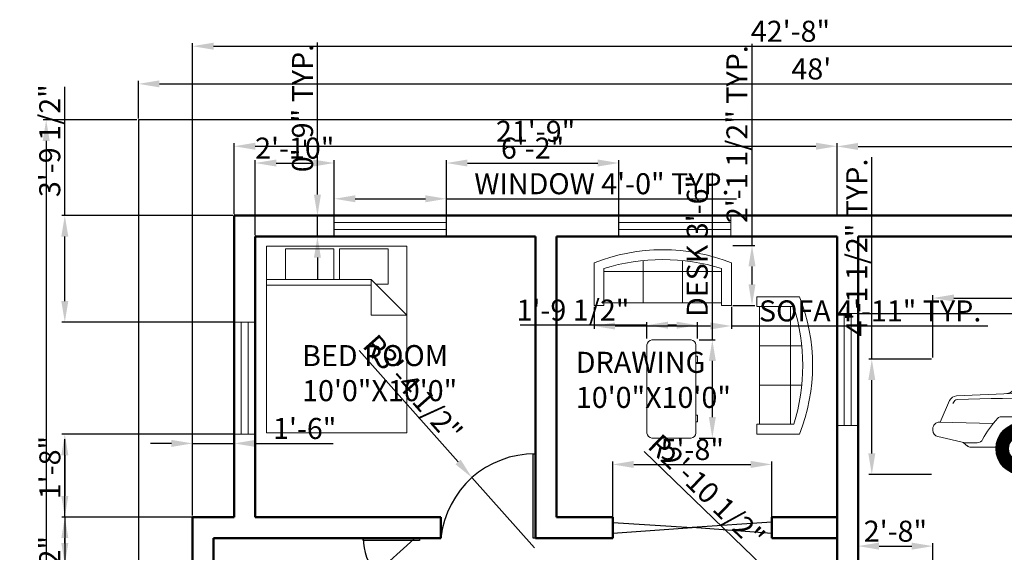
# Model space of a CAD drawing. Units: inches. Extents: x 2059616 to 2060276, y 889994 to 890582.
# Tile 3 of 4: x 2059616 to 2060037, y 890354 to 890582. Entities that reach past the tile are written whole.
import ezdxf

# ---------------------------------------------------------------- set-up
doc = ezdxf.new("R2010")
doc.units = ezdxf.units.IN
for name, color, linetype, lineweight in [('A-ANNO-DIMS', 2, 'Continuous', 18), ('A-AREA-IDEN', 7, 'Continuous', 25), ('A-DOOR', 3, 'Continuous', 25), ('A-FURN', 8, 'Continuous', 18), ('A-GLAZ', 4, 'Continuous', 18), ('A-SITE-VEHC', 8, 'Continuous', 18), ('A-WALL', 7, 'Continuous', 50), ('C-PROP', 7, 'Continuous', 25)]:
    doc.layers.add(name, color=color, linetype=linetype, lineweight=lineweight)
doc.styles.get("Standard").update_dxf_attribs({"font": 'arial.ttf'})
doc.dimstyles.new('ISO-25', dxfattribs={"dimtxt": 9, "dimasz": 9, "dimexe": 1.25, "dimexo": 0.625, "dimtad": 1, "dimdec": 1, "dimrnd": 9, "dimlunit": 3, "dimtxsty": 'Standard', "dimcen": 2.5, "dimadec": 0, "dimazin": 0, "dimtfac": 1, "dimtdec": 1, "dimtmove": 0, "dimatfit": 3, "dimfxl": 1, "dimarcsym": 0})

# ---------------------------------------------------------------- blocks, each defined once
blk = doc.blocks.new('*D1')
at = {"layer": 'A-ANNO-DIMS', "color": 0, "lineweight": -2, "transparency": 16777216}
for p, q in [((2059666.76, 890539.47), (2059666.76, 890555.48)), ((2059675.76, 890554.23), (2060233.76, 890554.23)), ((2060242.76, 890539.47), (2060242.76, 890555.48))]:
    blk.add_line(p, q, dxfattribs=at)
at = {"layer": 'A-ANNO-DIMS', "color": 0, "transparency": 16777216}
for points in [[(2059675.76, 890555.73), (2059675.76, 890552.73), (2059666.76, 890554.23)], [(2060233.76, 890555.73), (2060233.76, 890552.73), (2060242.76, 890554.23)]]:
    blk.add_solid(points, dxfattribs=at)
at = {"layer": 'Defpoints', "color": 0, "transparency": 16777216}
for p in [(2060242.76, 890554.23), (2059666.76, 890538.85), (2060242.76, 890538.85)]:
    blk.add_point(p, dxfattribs=at)
at = {"layer": 'A-ANNO-DIMS', "color": 0, "transparency": 16777216, "insert": (2059954.76, 890559.45), "char_height": 9, "attachment_point": 5}
blk.add_mtext("48'", dxfattribs=at)
blk = doc.blocks.new('*D2')
at = {"layer": 'A-ANNO-DIMS', "color": 0, "lineweight": -2, "transparency": 16777216}
for p, q in [((2059666.14, 890538.85), (2059626.05, 890538.85)), ((2059627.3, 890529.85), (2059627.3, 890091.85)), ((2059666.14, 890082.85), (2059626.05, 890082.85))]:
    blk.add_line(p, q, dxfattribs=at)
at = {"layer": 'A-ANNO-DIMS', "color": 0, "transparency": 16777216}
for points in [[(2059625.8, 890529.85), (2059628.8, 890529.85), (2059627.3, 890538.85)], [(2059625.8, 890091.85), (2059628.8, 890091.85), (2059627.3, 890082.85)]]:
    blk.add_solid(points, dxfattribs=at)
at = {"layer": 'Defpoints', "color": 0, "transparency": 16777216}
for p in [(2059666.76, 890538.85), (2059627.3, 890082.85), (2059666.76, 890082.85)]:
    blk.add_point(p, dxfattribs=at)
at = {"layer": 'A-ANNO-DIMS', "color": 0, "transparency": 16777216, "insert": (2059622.08, 890310.85), "char_height": 9, "attachment_point": 5, "rotation": 90}
blk.add_mtext('38\'-3"', dxfattribs=at)
blk = doc.blocks.new('Car - sedan  side')
for p, q in [((-139.53, 35.99), (-129.64, 47.91)), ((-128.57, 32.64), (-121.22, 48.02)), ((-77.81, 49.34), (-126.58, 49.34)), ((-74.7, 48.02), (-121.22, 48.02)), ((-120.32, 34.67), (-115.67, 48.02)), ((-115.4, 34.67), (-111.74, 48.02)), ((-97.55, 47.3), (-111.94, 47.3)), ((-94.41, 34.67), (-97.73, 48.02)), ((-93.72, 34.67), (-97.04, 48.02)), ((-93.03, 34.67), (-96.34, 48.02)), ((-76.26, 47.3), (-96.16, 47.3)), ((-61.08, 34.66), (-76.26, 47.3)), ((-60.02, 34.65), (-76.07, 48.02)), ((-56.87, 35.13), (-75.48, 48.59)), ((-58.54, 34.93), (-74.99, 48.02)), ((-140.23, 34.67), (-163.88, 33.56)), ((-62.28, 34.67), (-140.23, 34.67)), ((-93.72, 19.62), (-93.72, 34.67)), ((-62.28, 34.67), (-60.02, 34.65)), ((-60.02, 34.65), (-58.54, 34.93)), ((-57.97, 31.61), (-60.02, 34.65)), ((-57.21, 35.38), (-58.54, 34.93)), ((-54.93, 34.4), (-8.75, 29.8)), ((-170.93, 22.32), (-166.81, 31.56)), ((-164.57, 31.6), (-165.48, 30.35)), ((-130.39, 24.63), (-128.57, 32.64)), ((-57.97, 19.62), (-57.97, 31.61)), ((-4.21, 24.18), (-5.42, 27.27)), ((-148.26, 21.7), (-171.11, 22.33)), ((-128.78, 24.63), (-144.79, 24.63)), ((-36.97, 24.38), (-34.94, 24.38)), ((-174, 19.51), (-174, 18.91)), ((-47.2, 19.62), (-125.23, 19.62)), ((-93.72, 12.14), (-93.72, 19.62)), ((-57.97, 12.14), (-57.97, 19.62)), ((0, 19.62), (-24.7, 19.62)), ((-160.12, 13.48), (-171.81, 16.16)), ((-159.22, 12.14), (-161.08, 13.7)), ((-155.01, 13.48), (-160.12, 13.48)), ((-51.4, 9.89), (-49.69, 15.14)), ((-4.23, 13.19), (-20.72, 13.19)), ((-9.5, 13.19), (-14.1, 10.2)), ((-3.22, 13.59), (-1.77, 14.97)), ((-147.03, 11.6), (-157.73, 11.6)), ((-120.62, 9.03), (-125.23, 9.03)), ((-50.67, 12.14), (-123.32, 12.14)), ((-45.76, 9.03), (-120.62, 9.03)), ((-94.21, 9.03), (-94.21, 12.14)), ((-58.39, 9.03), (-58.39, 12.14)), ((-20.36, 11.06), (-24.06, 9.44)), ((-18.83, 10.42), (-19.11, 10.76)), ((-14.68, 10.03), (-18.01, 10.03))]:
    blk.add_line(p, q)
at = {"const_width": 5.49}
for points in [[(-127.8, 11, -1), (-144.3, 11, -1)], [(-26.69, 11, -1), (-43.19, 11, -1)]]:
    blk.add_lwpolyline(points, format="xyb", close=True, dxfattribs=at)
for centre, radius in [((-136.05, 11), 11), ((-34.94, 11), 11), ((-136.05, 11), 5.51), ((-34.94, 11), 5.51)]:
    blk.add_circle(centre, radius)
for centre, radius, start, end in [((-126.58, 45.38), 3.97, 90, 140.3029), ((-77.81, 45.38), 3.97, 54.135, 90), ((-142.58, 38.53), 3.97, 272.6827, 320.3029), ((-54.54, 38.35), 3.97, 234.135, 264.3123), ((-163.72, 30.18), 3.38, 92.6827, 155.9736), ((-163.62, 30.91), 1.17, 91.491, 143.9553), ((-118.51, -1702.12), 1734.79, 86.34698, 91.49105), ((-9.15, 25.82), 4, 21.3107, 84.3123), ((-171.18, 19.51), 2.82, 88.4193, 180), ((-118.09, -2.78), 38.85, 136.3964, 152.9097), ((-144.79, 22.64), 1.98, 90, 136.3964), ((-128.78, 22.64), 1.98, 28.1371, 90), ((-157.14, 7.48), 34.14, 6.5135, 28.1371), ((-36.97, 11), 13.38, 90, 161.9732), ((-34.94, 11), 13.38, 13.5864, 90), ((0.9, 26.18), 5.49, 201.3107, 247.7048), ((-1.92, 19.3), 1.94, 325.3744, 67.7048), ((-171.18, 18.91), 2.82, 180, 257.0905), ((2.46, 16.28), 3.37, 145.3744, 172.3839), ((-155.01, 16.1), 2.62, 270, 332.9097), ((-20.72, 14.43), 1.24, 193.5864, 270), ((-4.23, 14.65), 1.46, 270, 313.7173), ((-3.82, 17.12), 2.96, 313.7173, 352.3839), ((-157.73, 13.93), 2.32, 230.1291, 270), ((-120.62, 11.65), 2.62, 186.5135, 270), ((-52.58, 10.27), 1.24, 270, 341.9732), ((-19.93, 10.09), 1.06, 39.301, 113.7159), ((-18.01, 11.09), 1.06, 219.301, 270), ((-14.68, 11.09), 1.06, 270, 303.047)]:
    blk.add_arc(centre, radius, start, end)
blk = doc.blocks.new('Bed - Queen')
for p, q in [((0, -80.00003), (0, 0)), ((0, 0), (59.99999, 0)), ((59.99999, 0), (59.99999, -80.00003)), ((7.99999, -1.2), (28.79998, -1.2)), ((7.99999, -14.4), (7.99999, -1.2)), ((28.79998, -1.2), (28.79998, -14.4)), ((31.19999, -1.2), (51.99999, -1.2)), ((31.19999, -14.4), (31.19999, -1.2)), ((51.99999, -1.2), (51.99999, -16.4)), ((0, -14.4), (44.8, -14.4)), ((44.8, -16.8), (0, -16.8)), ((59.99999, -29.6), (44.8, -14.4)), ((44.8, -14.4), (44.8, -29.6)), ((51.99999, -16.4), (46.79936, -16.4)), ((44.8, -29.6), (59.99999, -29.6)), ((59.99999, -80.00003), (0, -80.00003))]:
    blk.add_line(p, q)
blk = doc.blocks.new('Sofa - Roundback 7 ft.')
for p, q in [((-36.000027, -34), (-36.000027, -11.4696)), ((-12.00002, -32.4421), (-12.00003, -6.5971)), ((11.99997, -32.4421), (11.99998, -6.5971)), ((35.99998, -34), (35.99998, -11.4696)), ((-35.999844, -13.3819), (35.9998, -13.3819)), ((-36.000027, -32.4421), (35.99998, -32.4421))]:
    blk.add_line(p, q)
for points in [[(-36.000027, -34), (-42.000027, -34), (-42.000027, -8)], [(41.99998, -8), (41.99998, -34), (35.99998, -34)]]:
    blk.add_lwpolyline(points)
for centre, radius, start, end in [((0, -114.25), 114.25, 68.43141, 111.5686), ((-0.00001, -127.1968), 121.1968, 72.72033, 107.2797)]:
    blk.add_arc(centre, radius, start, end)
blk = doc.blocks.new('Desk - 30 x 60 in.')
for p, q in [((-26.999995, 0), (26.999995, 0)), ((-29.999995, -27), (-29.999995, -3)), ((29.999995, -3), (29.999995, -27)), ((26.999995, -30), (-26.999995, -30)), ((-20.000005, -30), (-20.000005, -31)), ((-16.000005, -31), (-16.000005, -30)), ((15.999995, -31), (15.999995, -30)), ((19.999995, -30), (19.999995, -31)), ((-20.000005, -31), (-16.000005, -31)), ((19.999995, -31), (15.999995, -31))]:
    blk.add_line(p, q)
for centre, start, end in [((-26.499995, -3.5), 98.1301, 171.8699), ((26.499995, -3.5), 8.130102, 81.8699), ((-26.499995, -26.5), 188.1301, 261.8699), ((26.499995, -26.5), 278.1301, 351.8699)]:
    blk.add_arc(centre, 3.535534, start, end)
blk = doc.blocks.new('*D12')
at = {"layer": 'A-ANNO-DIMS', "color": 0, "lineweight": -2, "transparency": 16777216}
for p, q in [((2059707.76, 890498.47), (2059707.76, 890528.79)), ((2059965.76, 890498.47), (2059965.76, 890528.79)), ((2059716.76, 890527.54), (2059956.76, 890527.54))]:
    blk.add_line(p, q, dxfattribs=at)
at = {"layer": 'A-ANNO-DIMS', "color": 0, "transparency": 16777216}
for points in [[(2059716.76, 890529.04), (2059716.76, 890526.04), (2059707.76, 890527.54)], [(2059956.76, 890529.04), (2059956.76, 890526.04), (2059965.76, 890527.54)]]:
    blk.add_solid(points, dxfattribs=at)
at = {"layer": 'Defpoints', "color": 0, "transparency": 16777216}
for p in [(2059965.76, 890527.54), (2059707.76, 890497.85), (2059965.76, 890497.85)]:
    blk.add_point(p, dxfattribs=at)
at = {"layer": 'A-ANNO-DIMS', "color": 0, "transparency": 16777216, "insert": (2059836.76, 890532.76), "char_height": 9, "attachment_point": 5}
blk.add_mtext('21\'-9"', dxfattribs=at)
blk = doc.blocks.new('*D13')
at = {"layer": 'A-ANNO-DIMS', "color": 0, "lineweight": -2, "transparency": 16777216}
for p, q in [((2059965.76, 890498.47), (2059965.76, 890528.71)), ((2059974.76, 890527.46), (2060192.76, 890527.46)), ((2060201.76, 890498.47), (2060201.76, 890528.71))]:
    blk.add_line(p, q, dxfattribs=at)
at = {"layer": 'A-ANNO-DIMS', "color": 0, "transparency": 16777216}
for points in [[(2059974.76, 890528.96), (2059974.76, 890525.96), (2059965.76, 890527.46)], [(2060192.76, 890528.96), (2060192.76, 890525.96), (2060201.76, 890527.46)]]:
    blk.add_solid(points, dxfattribs=at)
at = {"layer": 'Defpoints', "color": 0, "transparency": 16777216}
for p in [(2060201.76, 890527.46), (2059965.76, 890497.85), (2060201.76, 890497.85)]:
    blk.add_point(p, dxfattribs=at)
at = {"layer": 'A-ANNO-DIMS', "color": 0, "transparency": 16777216, "insert": (2060083.76, 890532.68), "char_height": 9, "attachment_point": 5}
blk.add_mtext('19\'-6"', dxfattribs=at)
blk = doc.blocks.new('WIN-48IN')
for p, q in [((0, 9), (0, 0)), ((48, 9), (48, 0)), ((48, 6), (0, 6)), ((48, 3), (0, 3))]:
    blk.add_line(p, q)
blk = doc.blocks.new('*D16')
at = {"layer": 'A-ANNO-DIMS', "color": 0, "lineweight": -2, "transparency": 16777216}
for p, q in [((2059750.58, 890498.47), (2059750.58, 890506.3)), ((2059759.58, 890505.05), (2059789.58, 890505.05)), ((2059798.58, 890498.47), (2059798.58, 890506.3)), ((2059798.58, 890505.05), (2059922.72, 890505.05))]:
    blk.add_line(p, q, dxfattribs=at)
at = {"layer": 'A-ANNO-DIMS', "color": 0, "transparency": 16777216}
for points in [[(2059759.58, 890506.55), (2059759.58, 890503.55), (2059750.58, 890505.05)], [(2059789.58, 890506.55), (2059789.58, 890503.55), (2059798.58, 890505.05)]]:
    blk.add_solid(points, dxfattribs=at)
at = {"layer": 'Defpoints', "color": 0, "transparency": 16777216}
for p in [(2059798.58, 890505.05), (2059750.58, 890497.85), (2059798.58, 890497.85)]:
    blk.add_point(p, dxfattribs=at)
at = {"layer": 'A-ANNO-DIMS', "color": 0, "transparency": 16777216, "insert": (2059865.15, 890510.33), "char_height": 9, "attachment_point": 5}
blk.add_mtext('WINDOW 4\'-0" TYP.', dxfattribs=at)
blk = doc.blocks.new('*D17')
at = {"layer": 'A-ANNO-DIMS', "color": 0, "lineweight": -2, "transparency": 16777216}
for p, q in [((2059743.38, 890506.85), (2059743.38, 890571.96)), ((2059749.95, 890497.85), (2059742.13, 890497.85)), ((2059743.38, 890488.85), (2059743.38, 890497.85)), ((2059749.95, 890488.85), (2059742.13, 890488.85)), ((2059743.38, 890479.85), (2059743.38, 890470.85))]:
    blk.add_line(p, q, dxfattribs=at)
at = {"layer": 'A-ANNO-DIMS', "color": 0, "transparency": 16777216}
for points in [[(2059741.88, 890506.85), (2059744.88, 890506.85), (2059743.38, 890497.85)], [(2059741.88, 890479.85), (2059744.88, 890479.85), (2059743.38, 890488.85)]]:
    blk.add_solid(points, dxfattribs=at)
at = {"layer": 'Defpoints', "color": 0, "transparency": 16777216}
for p in [(2059743.38, 890497.85), (2059750.58, 890497.85), (2059750.58, 890488.85)]:
    blk.add_point(p, dxfattribs=at)
at = {"layer": 'A-ANNO-DIMS', "color": 0, "transparency": 16777216, "insert": (2059738.16, 890543.9), "char_height": 9, "attachment_point": 5, "rotation": 90}
blk.add_mtext('0\'-9" TYP.', dxfattribs=at)
blk = doc.blocks.new('*D20')
at = {"layer": 'A-ANNO-DIMS', "color": 0, "lineweight": -2, "transparency": 16777216}
for p, q in [((2060006.77, 890437.07), (2060006.77, 890463.82)), ((2060015.77, 890462.57), (2060171.88, 890462.57)), ((2060180.88, 890437.07), (2060180.88, 890463.82))]:
    blk.add_line(p, q, dxfattribs=at)
at = {"layer": 'A-ANNO-DIMS', "color": 0, "transparency": 16777216}
for points in [[(2060015.77, 890464.07), (2060015.77, 890461.07), (2060006.77, 890462.57)], [(2060171.88, 890464.07), (2060171.88, 890461.07), (2060180.88, 890462.57)]]:
    blk.add_solid(points, dxfattribs=at)
at = {"layer": 'Defpoints', "color": 0, "transparency": 16777216}
for p in [(2060180.88, 890462.57), (2060006.77, 890436.45), (2060180.88, 890436.45)]:
    blk.add_point(p, dxfattribs=at)
at = {"layer": 'A-ANNO-DIMS', "color": 0, "transparency": 16777216, "insert": (2060093.82, 890467.84), "char_height": 9, "attachment_point": 5}
blk.add_mtext('SEDAN 14\'-6" TYP.', dxfattribs=at)
blk = doc.blocks.new('*D21')
at = {"layer": 'A-ANNO-DIMS', "color": 0, "lineweight": -2, "transparency": 16777216}
for p, q in [((2059980.65, 890436.45), (2059980.65, 890522.89)), ((2060006.14, 890436.45), (2059979.4, 890436.45)), ((2059980.65, 890396.1), (2059980.65, 890427.45)), ((2060006.14, 890387.1), (2059979.4, 890387.1))]:
    blk.add_line(p, q, dxfattribs=at)
at = {"layer": 'A-ANNO-DIMS', "color": 0, "transparency": 16777216}
for points in [[(2059979.15, 890427.45), (2059982.15, 890427.45), (2059980.65, 890436.45)], [(2059979.15, 890396.1), (2059982.15, 890396.1), (2059980.65, 890387.1)]]:
    blk.add_solid(points, dxfattribs=at)
at = {"layer": 'Defpoints', "color": 0, "transparency": 16777216}
for p in [(2059980.65, 890436.45), (2060006.77, 890436.45), (2060006.77, 890387.1)]:
    blk.add_point(p, dxfattribs=at)
at = {"layer": 'A-ANNO-DIMS', "color": 0, "transparency": 16777216, "insert": (2059975.37, 890484.17), "char_height": 9, "attachment_point": 5, "rotation": 90}
blk.add_mtext('4\'-1 1/2" TYP.', dxfattribs=at)
blk = doc.blocks.new('*D26')
at = {"layer": 'A-ANNO-DIMS', "color": 0, "lineweight": -2, "transparency": 16777216}
for p, q in [((2059861.76, 890458.81), (2059861.76, 890449.36)), ((2059920.56, 890458.81), (2059920.56, 890449.36)), ((2059870.76, 890450.61), (2059911.56, 890450.61)), ((2059920.56, 890450.61), (2060030.34, 890450.61))]:
    blk.add_line(p, q, dxfattribs=at)
at = {"layer": 'A-ANNO-DIMS', "color": 0, "transparency": 16777216}
for points in [[(2059870.76, 890452.11), (2059870.76, 890449.11), (2059861.76, 890450.61)], [(2059911.56, 890452.11), (2059911.56, 890449.11), (2059920.56, 890450.61)]]:
    blk.add_solid(points, dxfattribs=at)
at = {"layer": 'Defpoints', "color": 0, "transparency": 16777216}
for p in [(2059861.76, 890459.43), (2059920.56, 890459.43), (2059920.56, 890450.61)]:
    blk.add_point(p, dxfattribs=at)
at = {"layer": 'A-ANNO-DIMS', "color": 0, "transparency": 16777216, "insert": (2059979.95, 890455.9), "char_height": 9, "attachment_point": 5}
blk.add_mtext('SOFA 4\'-11" TYP.', dxfattribs=at)
blk = doc.blocks.new('*D27')
at = {"layer": 'A-ANNO-DIMS', "color": 0, "lineweight": -2, "transparency": 16777216}
for p, q in [((2059929.38, 890485.1), (2059929.38, 890571.34)), ((2059921.19, 890485.1), (2059930.63, 890485.1)), ((2059929.38, 890468.43), (2059929.38, 890476.1)), ((2059921.19, 890459.43), (2059930.63, 890459.43))]:
    blk.add_line(p, q, dxfattribs=at)
at = {"layer": 'A-ANNO-DIMS', "color": 0, "transparency": 16777216}
for points in [[(2059927.88, 890476.1), (2059930.88, 890476.1), (2059929.38, 890485.1)], [(2059927.88, 890468.43), (2059930.88, 890468.43), (2059929.38, 890459.43)]]:
    blk.add_solid(points, dxfattribs=at)
at = {"layer": 'Defpoints', "color": 0, "transparency": 16777216}
for p in [(2059920.56, 890485.1), (2059929.38, 890485.1), (2059920.56, 890459.43)]:
    blk.add_point(p, dxfattribs=at)
at = {"layer": 'A-ANNO-DIMS', "color": 0, "transparency": 16777216, "insert": (2059924.1, 890532.72), "char_height": 9, "attachment_point": 5, "rotation": 90}
blk.add_mtext('2\'-1 1/2" TYP.', dxfattribs=at)
blk = doc.blocks.new('*D30')
at = {"layer": 'A-ANNO-DIMS', "color": 0, "lineweight": -2, "transparency": 16777216}
for p, q in [((2059912.4, 890444.64), (2059912.4, 890516.09)), ((2059906.73, 890444.64), (2059913.65, 890444.64)), ((2059912.4, 890411.64), (2059912.4, 890435.64)), ((2059906.73, 890402.64), (2059913.65, 890402.64))]:
    blk.add_line(p, q, dxfattribs=at)
at = {"layer": 'A-ANNO-DIMS', "color": 0, "transparency": 16777216}
for points in [[(2059910.9, 890435.64), (2059913.9, 890435.64), (2059912.4, 890444.64)], [(2059910.9, 890411.64), (2059913.9, 890411.64), (2059912.4, 890402.64)]]:
    blk.add_solid(points, dxfattribs=at)
at = {"layer": 'Defpoints', "color": 0, "transparency": 16777216}
for p in [(2059906.1, 890444.64), (2059912.4, 890444.64), (2059906.1, 890402.64)]:
    blk.add_point(p, dxfattribs=at)
at = {"layer": 'A-ANNO-DIMS', "color": 0, "transparency": 16777216, "insert": (2059907.12, 890484.87), "char_height": 9, "attachment_point": 5, "rotation": 90}
blk.add_mtext('DESK 3\'-6"', dxfattribs=at)
blk = doc.blocks.new('*D31')
at = {"layer": 'A-ANNO-DIMS', "color": 0, "lineweight": -2, "transparency": 16777216}
for p, q in [((2059884.4, 890450.94), (2059830.1, 890450.94)), ((2059884.4, 890445.26), (2059884.4, 890452.19)), ((2059897.1, 890450.94), (2059893.4, 890450.94)), ((2059906.1, 890445.26), (2059906.1, 890452.19))]:
    blk.add_line(p, q, dxfattribs=at)
at = {"layer": 'A-ANNO-DIMS', "color": 0, "transparency": 16777216}
for points in [[(2059893.4, 890452.44), (2059893.4, 890449.44), (2059884.4, 890450.94)], [(2059897.1, 890452.44), (2059897.1, 890449.44), (2059906.1, 890450.94)]]:
    blk.add_solid(points, dxfattribs=at)
at = {"layer": 'Defpoints', "color": 0, "transparency": 16777216}
for p in [(2059884.4, 890450.94), (2059884.4, 890444.64), (2059906.1, 890444.64)]:
    blk.add_point(p, dxfattribs=at)
at = {"layer": 'A-ANNO-DIMS', "color": 0, "transparency": 16777216, "insert": (2059852.75, 890456.22), "char_height": 9, "attachment_point": 5}
blk.add_mtext('1\'-9 1/2"', dxfattribs=at)
blk = doc.blocks.new('*D38')
at = {"layer": 'A-ANNO-DIMS', "color": 0, "lineweight": -2, "transparency": 16777216}
for p, q in [((2059689.91, 890369.47), (2059689.91, 890571.6)), ((2060201.76, 890498.47), (2060201.76, 890571.6)), ((2059698.91, 890570.35), (2060192.76, 890570.35))]:
    blk.add_line(p, q, dxfattribs=at)
at = {"layer": 'A-ANNO-DIMS', "color": 0, "transparency": 16777216}
for points in [[(2059698.91, 890571.85), (2059698.91, 890568.85), (2059689.91, 890570.35)], [(2060192.76, 890571.85), (2060192.76, 890568.85), (2060201.76, 890570.35)]]:
    blk.add_solid(points, dxfattribs=at)
at = {"layer": 'Defpoints', "color": 0, "transparency": 16777216}
for p in [(2060201.76, 890570.35), (2060201.76, 890497.85), (2059689.91, 890368.85)]:
    blk.add_point(p, dxfattribs=at)
at = {"layer": 'A-ANNO-DIMS', "color": 0, "transparency": 16777216, "insert": (2059945.84, 890575.57), "char_height": 9, "attachment_point": 5}
blk.add_mtext('42\'-8"', dxfattribs=at)
blk = doc.blocks.new('*D39')
at = {"layer": 'A-ANNO-DIMS', "color": 0, "lineweight": -2, "transparency": 16777216}
for p, q in [((2060202.39, 890497.85), (2060275.51, 890497.85)), ((2060274.26, 890127.85), (2060274.26, 890488.85)), ((2059926.39, 890118.85), (2060275.51, 890118.85))]:
    blk.add_line(p, q, dxfattribs=at)
at = {"layer": 'A-ANNO-DIMS', "color": 0, "transparency": 16777216}
for points in [[(2060272.76, 890488.85), (2060275.76, 890488.85), (2060274.26, 890497.85)], [(2060272.76, 890127.85), (2060275.76, 890127.85), (2060274.26, 890118.85)]]:
    blk.add_solid(points, dxfattribs=at)
at = {"layer": 'Defpoints', "color": 0, "transparency": 16777216}
for p in [(2060201.76, 890497.85), (2060274.26, 890497.85), (2059925.76, 890118.85)]:
    blk.add_point(p, dxfattribs=at)
at = {"layer": 'A-ANNO-DIMS', "color": 0, "transparency": 16777216, "insert": (2060269.04, 890308.35), "char_height": 9, "attachment_point": 5, "rotation": 90}
blk.add_mtext('31\'-7"', dxfattribs=at)
blk = doc.blocks.new('*D40')
at = {"layer": 'A-ANNO-DIMS', "color": 0, "lineweight": -2, "transparency": 16777216}
for p, q in [((2059707.14, 890404.26), (2059634.01, 890404.26)), ((2059635.26, 890395.26), (2059635.26, 890377.85)), ((2059707.14, 890368.85), (2059634.01, 890368.85)), ((2059635.26, 890368.85), (2059635.26, 890306.55))]:
    blk.add_line(p, q, dxfattribs=at)
at = {"layer": 'A-ANNO-DIMS', "color": 0, "transparency": 16777216}
for points in [[(2059633.76, 890395.26), (2059636.76, 890395.26), (2059635.26, 890404.26)], [(2059633.76, 890377.85), (2059636.76, 890377.85), (2059635.26, 890368.85)]]:
    blk.add_solid(points, dxfattribs=at)
at = {"layer": 'Defpoints', "color": 0, "transparency": 16777216}
for p in [(2059707.76, 890404.26), (2059635.26, 890368.85), (2059707.76, 890368.85)]:
    blk.add_point(p, dxfattribs=at)
at = {"layer": 'A-ANNO-DIMS', "color": 0, "transparency": 16777216, "insert": (2059629.98, 890333.2), "char_height": 9, "attachment_point": 5, "rotation": 90}
blk.add_mtext('2\'-11 1/2"', dxfattribs=at)
blk = doc.blocks.new('*D42')
at = {"layer": 'A-ANNO-DIMS', "color": 0, "lineweight": -2, "transparency": 16777216}
for p, q in [((2059680.91, 890400.35), (2059671.91, 890400.35)), ((2059689.91, 890369.47), (2059689.91, 890401.6)), ((2059689.91, 890400.35), (2059707.76, 890400.35)), ((2059707.76, 890369.47), (2059707.76, 890401.6)), ((2059716.76, 890400.35), (2059750.09, 890400.35))]:
    blk.add_line(p, q, dxfattribs=at)
at = {"layer": 'A-ANNO-DIMS', "color": 0, "transparency": 16777216}
for points in [[(2059680.91, 890401.85), (2059680.91, 890398.85), (2059689.91, 890400.35)], [(2059716.76, 890401.85), (2059716.76, 890398.85), (2059707.76, 890400.35)]]:
    blk.add_solid(points, dxfattribs=at)
at = {"layer": 'Defpoints', "color": 0, "transparency": 16777216}
for p in [(2059707.76, 890400.35), (2059689.91, 890368.85), (2059707.76, 890368.85)]:
    blk.add_point(p, dxfattribs=at)
at = {"layer": 'A-ANNO-DIMS', "color": 0, "transparency": 16777216, "insert": (2059737.93, 890405.57), "char_height": 9, "attachment_point": 5}
blk.add_mtext('1\'-6"', dxfattribs=at)
blk = doc.blocks.new('*D45')
at = {"layer": 'A-ANNO-DIMS', "color": 0, "lineweight": -2, "transparency": 16777216}
for p, q in [((2059716.76, 890489.47), (2059716.76, 890521.6)), ((2059750.58, 890489.47), (2059750.58, 890521.6)), ((2059725.76, 890520.35), (2059741.58, 890520.35))]:
    blk.add_line(p, q, dxfattribs=at)
at = {"layer": 'A-ANNO-DIMS', "color": 0, "transparency": 16777216}
for points in [[(2059725.76, 890521.85), (2059725.76, 890518.85), (2059716.76, 890520.35)], [(2059741.58, 890521.85), (2059741.58, 890518.85), (2059750.58, 890520.35)]]:
    blk.add_solid(points, dxfattribs=at)
at = {"layer": 'Defpoints', "color": 0, "transparency": 16777216}
for p in [(2059750.58, 890520.35), (2059716.76, 890488.85), (2059750.58, 890488.85)]:
    blk.add_point(p, dxfattribs=at)
at = {"layer": 'A-ANNO-DIMS', "color": 0, "transparency": 16777216, "insert": (2059733.67, 890525.57), "char_height": 9, "attachment_point": 5}
blk.add_mtext('2\'-10"', dxfattribs=at)
blk = doc.blocks.new('*D46')
at = {"layer": 'A-ANNO-DIMS', "color": 0, "lineweight": -2, "transparency": 16777216}
for p, q in [((2059798.58, 890489.47), (2059798.58, 890521.6)), ((2059872.33, 890489.47), (2059872.33, 890521.6)), ((2059807.58, 890520.35), (2059863.33, 890520.35))]:
    blk.add_line(p, q, dxfattribs=at)
at = {"layer": 'A-ANNO-DIMS', "color": 0, "transparency": 16777216}
for points in [[(2059807.58, 890521.85), (2059807.58, 890518.85), (2059798.58, 890520.35)], [(2059863.33, 890521.85), (2059863.33, 890518.85), (2059872.33, 890520.35)]]:
    blk.add_solid(points, dxfattribs=at)
at = {"layer": 'Defpoints', "color": 0, "transparency": 16777216}
for p in [(2059872.33, 890520.35), (2059798.58, 890488.85), (2059872.33, 890488.85)]:
    blk.add_point(p, dxfattribs=at)
at = {"layer": 'A-ANNO-DIMS', "color": 0, "transparency": 16777216, "insert": (2059835.46, 890525.57), "char_height": 9, "attachment_point": 5}
blk.add_mtext('6\'-2"', dxfattribs=at)
blk = doc.blocks.new('*D47')
at = {"layer": 'A-ANNO-DIMS', "color": 0, "lineweight": -2, "transparency": 16777216}
for p, q in [((2059635.26, 890497.85), (2059635.26, 890552.99)), ((2059707.14, 890497.85), (2059634.01, 890497.85)), ((2059635.26, 890461.26), (2059635.26, 890488.85)), ((2059707.14, 890452.26), (2059634.01, 890452.26))]:
    blk.add_line(p, q, dxfattribs=at)
at = {"layer": 'A-ANNO-DIMS', "color": 0, "transparency": 16777216}
for points in [[(2059633.76, 890488.85), (2059636.76, 890488.85), (2059635.26, 890497.85)], [(2059633.76, 890461.26), (2059636.76, 890461.26), (2059635.26, 890452.26)]]:
    blk.add_solid(points, dxfattribs=at)
at = {"layer": 'Defpoints', "color": 0, "transparency": 16777216}
for p in [(2059635.26, 890497.85), (2059707.76, 890497.85), (2059707.76, 890452.26)]:
    blk.add_point(p, dxfattribs=at)
at = {"layer": 'A-ANNO-DIMS', "color": 0, "transparency": 16777216, "insert": (2059629.98, 890529.92), "char_height": 9, "attachment_point": 5, "rotation": 90}
blk.add_mtext('3\'-9 1/2"', dxfattribs=at)
blk = doc.blocks.new('*D49')
at = {"layer": 'A-ANNO-DIMS', "color": 0, "lineweight": -2, "transparency": 16777216}
for p, q in [((2059635.26, 890368.85), (2059635.26, 890402.17)), ((2059689.29, 890368.85), (2059634.01, 890368.85)), ((2059635.26, 890357.68), (2059635.26, 890359.85)), ((2059689.29, 890348.68), (2059634.01, 890348.68))]:
    blk.add_line(p, q, dxfattribs=at)
at = {"layer": 'A-ANNO-DIMS', "color": 0, "transparency": 16777216}
for points in [[(2059633.76, 890359.85), (2059636.76, 890359.85), (2059635.26, 890368.85)], [(2059633.76, 890357.68), (2059636.76, 890357.68), (2059635.26, 890348.68)]]:
    blk.add_solid(points, dxfattribs=at)
at = {"layer": 'Defpoints', "color": 0, "transparency": 16777216}
for p in [(2059635.26, 890368.85), (2059689.91, 890368.85), (2059689.91, 890348.68)]:
    blk.add_point(p, dxfattribs=at)
at = {"layer": 'A-ANNO-DIMS', "color": 0, "transparency": 16777216, "insert": (2059630.04, 890390.01), "char_height": 9, "attachment_point": 5, "rotation": 90}
blk.add_mtext('1\'-8"', dxfattribs=at)
blk = doc.blocks.new('*D53')
at = {"layer": 'A-ANNO-DIMS', "color": 0, "lineweight": -2, "transparency": 16777216}
for p, q in [((2059975.39, 890488.85), (2060275.51, 890488.85)), ((2060274.26, 890464.97), (2060274.26, 890479.85)), ((2059975.39, 890455.97), (2060275.51, 890455.97))]:
    blk.add_line(p, q, dxfattribs=at)
at = {"layer": 'A-ANNO-DIMS', "color": 0, "transparency": 16777216}
for points in [[(2060272.76, 890479.85), (2060275.76, 890479.85), (2060274.26, 890488.85)], [(2060272.76, 890464.97), (2060275.76, 890464.97), (2060274.26, 890455.97)]]:
    blk.add_solid(points, dxfattribs=at)
at = {"layer": 'Defpoints', "color": 0, "transparency": 16777216}
for p in [(2059974.76, 890488.85), (2060274.26, 890488.85), (2059974.76, 890455.97)]:
    blk.add_point(p, dxfattribs=at)
at = {"layer": 'A-ANNO-DIMS', "color": 0, "transparency": 16777216, "insert": (2060269.04, 890472.41), "char_height": 9, "attachment_point": 5, "rotation": 90}
blk.add_mtext('2\'-9"', dxfattribs=at)
blk = doc.blocks.new('*D54')
at = {"layer": 'A-ANNO-DIMS', "color": 0, "lineweight": -2, "transparency": 16777216}
for p, q in [((2059974.76, 890325.51), (2059974.76, 890357.64)), ((2059983.76, 890356.39), (2059997.76, 890356.39)), ((2060006.76, 890325.51), (2060006.76, 890357.64))]:
    blk.add_line(p, q, dxfattribs=at)
at = {"layer": 'A-ANNO-DIMS', "color": 0, "transparency": 16777216}
for points in [[(2059983.76, 890357.89), (2059983.76, 890354.89), (2059974.76, 890356.39)], [(2059997.76, 890357.89), (2059997.76, 890354.89), (2060006.76, 890356.39)]]:
    blk.add_solid(points, dxfattribs=at)
at = {"layer": 'Defpoints', "color": 0, "transparency": 16777216}
for p in [(2060006.76, 890356.39), (2059974.76, 890324.89), (2060006.76, 890324.89)]:
    blk.add_point(p, dxfattribs=at)
at = {"layer": 'A-ANNO-DIMS', "color": 0, "transparency": 16777216, "insert": (2059990.76, 890361.61), "char_height": 9, "attachment_point": 5}
blk.add_mtext('2\'-8"', dxfattribs=at)
blk = doc.blocks.new('*D58')
at = {"layer": 'A-ANNO-DIMS', "color": 0, "lineweight": -2, "transparency": 16777216}
for p, q in [((2059869.76, 890360.47), (2059869.76, 890392.6)), ((2059878.76, 890391.35), (2059928.85, 890391.35)), ((2059937.85, 890360.47), (2059937.85, 890392.6))]:
    blk.add_line(p, q, dxfattribs=at)
at = {"layer": 'A-ANNO-DIMS', "color": 0, "transparency": 16777216}
for points in [[(2059878.76, 890392.85), (2059878.76, 890389.85), (2059869.76, 890391.35)], [(2059928.85, 890392.85), (2059928.85, 890389.85), (2059937.85, 890391.35)]]:
    blk.add_solid(points, dxfattribs=at)
at = {"layer": 'Defpoints', "color": 0, "transparency": 16777216}
for p in [(2059937.85, 890391.35), (2059869.76, 890359.85), (2059937.85, 890359.85)]:
    blk.add_point(p, dxfattribs=at)
at = {"layer": 'A-ANNO-DIMS', "color": 0, "transparency": 16777216, "insert": (2059903.81, 890396.57), "char_height": 9, "attachment_point": 5}
blk.add_mtext('5\'-8"', dxfattribs=at)
blk = doc.blocks.new('*D62')
at = {"layer": 'A-ANNO-DIMS', "color": 0, "lineweight": -2, "transparency": 16777216}
for p, q in [((2059761.21, 890440.09), (2059803.55, 890392.42)), ((2059836.26, 890355.59), (2059809.53, 890385.69))]:
    blk.add_line(p, q, dxfattribs=at)
at = {"layer": 'A-ANNO-DIMS', "color": 0, "transparency": 16777216}
blk.add_solid([(2059804.67, 890393.42), (2059802.43, 890391.42), (2059809.53, 890385.69)], dxfattribs=at)
at = {"layer": 'Defpoints', "color": 0, "transparency": 16777216}
for p in [(2059809.53, 890385.69), (2059836.26, 890355.59)]:
    blk.add_point(p, dxfattribs=at)
at = {"layer": 'A-ANNO-DIMS', "color": 0, "transparency": 16777216, "insert": (2059783.34, 890423.13), "char_height": 9, "attachment_point": 5, "rotation": 311.6088}
blk.add_mtext('R3\'-4 1/2"', dxfattribs=at)
blk = doc.blocks.new('*D63')
at = {"layer": 'A-ANNO-DIMS', "color": 0, "lineweight": -2, "transparency": 16777216}
for p, q in [((2059883.25, 890396.89), (2059934.09, 890347.68)), ((2059965.26, 890317.5), (2059940.56, 890341.42))]:
    blk.add_line(p, q, dxfattribs=at)
at = {"layer": 'A-ANNO-DIMS', "color": 0, "transparency": 16777216}
blk.add_solid([(2059935.13, 890348.76), (2059933.05, 890346.61), (2059940.56, 890341.42)], dxfattribs=at)
at = {"layer": 'Defpoints', "color": 0, "transparency": 16777216}
for p in [(2059940.56, 890341.42), (2059965.26, 890317.5)]:
    blk.add_point(p, dxfattribs=at)
at = {"layer": 'A-ANNO-DIMS', "color": 0, "transparency": 16777216, "insert": (2059909.11, 890379.21), "char_height": 9, "attachment_point": 5, "rotation": 315.9294}
blk.add_mtext('R2\'-10 1/2"', dxfattribs=at)
blk = doc.blocks.new('*D64')
at = {"layer": 'A-ANNO-DIMS', "color": 0, "lineweight": -2, "transparency": 16777216}
for p, q in [((2059784.66, 890359.35), (2059768.57, 890344.84)), ((2059714.52, 890296.13), (2059761.88, 890338.82))]:
    blk.add_line(p, q, dxfattribs=at)
at = {"layer": 'A-ANNO-DIMS', "color": 0, "transparency": 16777216}
blk.add_solid([(2059760.88, 890339.93), (2059762.89, 890337.7), (2059768.57, 890344.84)], dxfattribs=at)
at = {"layer": 'Defpoints', "color": 0, "transparency": 16777216}
for p in [(2059784.66, 890359.35), (2059768.57, 890344.84)]:
    blk.add_point(p, dxfattribs=at)
at = {"layer": 'A-ANNO-DIMS', "color": 0, "transparency": 16777216, "insert": (2059731.33, 890318.38), "char_height": 9, "attachment_point": 5, "rotation": 42.0332}
blk.add_mtext('R1\'-9 1/2"', dxfattribs=at)

msp = doc.modelspace()

# ---------------------------------------------------------------- linework, layer by layer
at = {"layer": 'A-DOOR'}
for p, q in [((2059835.76, 890359.85), (2059835.76, 890395.85)), ((2059835.76, 890395.85), (2059836.76, 890395.85)), ((2059869.76, 890366.48), (2059903.81, 890364.35)), ((2059937.85, 890366.62), (2059903.81, 890364.35)), ((2059869.76, 890361.97), (2059903.81, 890364.35)), ((2059937.85, 890361.82), (2059903.81, 890364.35)), ((2059763, 890358.85), (2059763, 890359.85)), ((2059787, 890358.85), (2059763, 890358.85)), ((2059787, 890359.85), (2059787, 890358.85)), ((2059836.76, 890359.85), (2059835.76, 890359.85))]:
    msp.add_line(p, q, dxfattribs=at)
for centre, radius, start, end in [((2059836.26, 890355.59), 40.26, 89.2884, 173.9294), ((2059784.66, 890359.35), 21.66, 178.6774, 265.3869)]:
    msp.add_arc(centre, radius, start, end, dxfattribs=at)
at = {"layer": 'A-WALL'}
for p, q in [((2059707.76, 890497.85), (2059707.76, 890368.85)), ((2060201.76, 890497.85), (2059707.76, 890497.85)), ((2059716.76, 890488.85), (2059716.76, 890368.85)), ((2059836.76, 890488.85), (2059716.76, 890488.85)), ((2059836.76, 890488.85), (2059836.76, 890359.85)), ((2059845.76, 890488.85), (2059845.76, 890368.85)), ((2059965.76, 890488.85), (2059845.76, 890488.85)), ((2059965.76, 890488.85), (2059965.76, 890315.89)), ((2060192.76, 890488.85), (2059974.76, 890488.85)), ((2059974.76, 890488.85), (2059974.76, 890324.89)), ((2059707.76, 890368.85), (2059689.91, 890368.85)), ((2059689.91, 890368.85), (2059689.91, 890359.85)), ((2059796.23, 890368.85), (2059716.76, 890368.85)), ((2059796.23, 890368.85), (2059796.23, 890359.85)), ((2059869.76, 890368.85), (2059845.76, 890368.85)), ((2059869.76, 890359.85), (2059869.76, 890368.85)), ((2059965.76, 890368.85), (2059937.85, 890368.85)), ((2059937.85, 890368.85), (2059937.85, 890359.85)), ((2059689.91, 890359.85), (2059689.91, 890259.85)), ((2059698.91, 890359.85), (2059698.91, 890314.35)), ((2059707.76, 890359.85), (2059698.91, 890359.85)), ((2059796.23, 890359.85), (2059707.76, 890359.85)), ((2059869.76, 890359.85), (2059836.76, 890359.85)), ((2059965.76, 890359.85), (2059937.85, 890359.85))]:
    msp.add_line(p, q, dxfattribs=at)
at = {"layer": 'C-PROP'}
for p, q in [((2060242.76, 890538.85), (2059666.76, 890538.85)), ((2059666.76, 890538.85), (2059666.76, 890082.85))]:
    msp.add_line(p, q, dxfattribs=at)

# ---------------------------------------------------------------- block references
at = {"layer": 'A-FURN'}
msp.add_blockref('Bed - Queen', (2059721.65, 890484.84), dxfattribs=at)
at = {"layer": 'A-FURN', "xscale": 0.7, "yscale": 0.7}
msp.add_blockref('Sofa - Roundback 7 ft.', (2059891.16, 890483.23), dxfattribs=at)
for name, p, rotation in [('Sofa - Roundback 7 ft.', (2059955.29, 890433.72), 270), ('Desk - 30 x 60 in.', (2059884.4, 890423.64), 90)]:
    msp.add_blockref(name, p, dxfattribs=dict(at, rotation=rotation))
at = {"layer": 'A-GLAZ'}
for p in [(2059750.58, 890488.85), (2059872.33, 890488.85)]:
    msp.add_blockref('WIN-48IN', p, dxfattribs=at)
for p, rotation in [((2059965.76, 890455.97), 270.0000000001174), ((2059707.76, 890452.26), 270.0000000000671)]:
    msp.add_blockref('WIN-48IN', p, dxfattribs=dict(at, rotation=rotation))
at = {"layer": 'A-SITE-VEHC'}
msp.add_blockref('Car - sedan  side', (2060180.77, 890387.1), dxfattribs=at)

# ---------------------------------------------------------------- texts
at = {"layer": 'A-AREA-IDEN', "char_height": 9, "attachment_point": 1}
for s, insert in [('BED ROOM\\P10\'0"X10\'0"', (2059736.82, 890442.43)), ('DRAWING\\P10\'0"X10\'0"', (2059853.97, 890439.55))]:
    msp.add_mtext_dynamic_manual_height_columns(s, width=69.4215, gutter_width=12.5, heights=[0], dxfattribs=dict(at, insert=insert))

# ---------------------------------------------------------------- dimensions: what is measured, and where the dimension line sits
at = {"layer": 'A-ANNO-DIMS'}
for base, p1, p2, override, picture, middle in [((2060201.7635, 890570.3463), (2059689.9147, 890368.8463), (2060201.7635, 890497.8463), {"dimdec": 1, "dimlfac": 1, "dimrnd": 0, "dimzin": 1, "dimdsep": 46, "dimlunit": 4, "dimfrac": 2}, '*D38', (2059945.8391, 890575.5665)), ((2060242.76, 890554.23), (2059666.76, 890538.85), (2060242.76, 890538.85), {"dimclrd": 0, "dimclre": 0, "dimclrt": 0}, '*D1', (2059954.76, 890559.45)), ((2059965.76, 890527.54), (2059707.76, 890497.85), (2059965.76, 890497.85), {"dimclrd": 0, "dimclre": 0, "dimclrt": 0}, '*D12', (2059836.76, 890532.76)), ((2060201.76, 890527.46), (2059965.76, 890497.85), (2060201.76, 890497.85), {"dimclrd": 0, "dimclre": 0, "dimclrt": 0}, '*D13', (2060083.76, 890532.68)), ((2059750.58, 890520.35), (2059716.76, 890488.85), (2059750.58, 890488.85), {"dimdec": 1, "dimlfac": 1, "dimrnd": 0, "dimzin": 1, "dimdsep": 46, "dimlunit": 4, "dimfrac": 2}, '*D45', (2059733.67, 890525.57)), ((2059872.3332, 890520.3463), (2059798.5783, 890488.8463), (2059872.3332, 890488.8463), {"dimdec": 1, "dimlfac": 1, "dimrnd": 0, "dimzin": 1, "dimdsep": 46, "dimlunit": 4, "dimfrac": 2}, '*D46', (2059835.4558, 890525.5665)), ((2059937.85, 890391.35), (2059869.76, 890359.85), (2059937.85, 890359.85), {"dimdec": 1, "dimlfac": 1, "dimrnd": 0, "dimzin": 1, "dimdsep": 46, "dimlunit": 4, "dimfrac": 2}, '*D58', (2059903.81, 890396.57)), ((2060006.76, 890356.39), (2059974.76, 890324.89), (2060006.76, 890324.89), {"dimdec": 1, "dimlfac": 1, "dimrnd": 0, "dimzin": 1, "dimdsep": 46, "dimlunit": 4, "dimfrac": 2}, '*D54', (2059990.76, 890361.61))]:
    dim = msp.add_linear_dim(base=base, p1=p1, p2=p2, dimstyle='ISO-25', override=override, dxfattribs=at)
    dim.commit()
    dim.dimension.update_dxf_attribs({"geometry": picture, "text_midpoint": middle})
for base, p1, p2, text, picture, middle in [((2059743.38, 890497.85), (2059750.58, 890488.85), (2059750.58, 890497.85), '<> TYP.', '*D17', (2059738.16, 890543.9)), ((2059929.38, 890485.1), (2059920.56, 890459.43), (2059920.56, 890485.1), '<> TYP.', '*D27', (2059924.1, 890532.72)), ((2059980.6495, 890436.449), (2060006.7666, 890387.1041), (2060006.7666, 890436.449), '<> TYP.', '*D21', (2059975.3711, 890484.1705)), ((2059912.4, 890444.64), (2059906.1, 890402.64), (2059906.1, 890444.64), 'DESK <>', '*D30', (2059907.12, 890484.87))]:
    dim = msp.add_linear_dim(base=base, p1=p1, p2=p2, angle=90, text=text, dimstyle='ISO-25', override={"dimdec": 1, "dimlfac": 1, "dimrnd": 0, "dimzin": 1, "dimdsep": 46, "dimlunit": 4, "dimfrac": 2}, dxfattribs=at)
    dim.commit()
    dim.dimension.update_dxf_attribs({"geometry": picture, "text_midpoint": middle})
for base, p1, p2, angle, override, picture, middle in [((2059635.26, 890497.85), (2059707.76, 890452.26), (2059707.76, 890497.85), 90, {"dimdec": 1, "dimlfac": 1, "dimrnd": 0, "dimzin": 1, "dimdsep": 46, "dimlunit": 4, "dimfrac": 2}, '*D47', (2059629.98, 890529.92)), ((2059627.3, 890082.85), (2059666.76, 890538.85), (2059666.76, 890082.85), 90, {"dimclrd": 0, "dimclre": 0, "dimclrt": 0}, '*D2', (2059622.08, 890310.85)), ((2060274.26, 890497.85), (2059925.76, 890118.85), (2060201.76, 890497.85), 90, {"dimdec": 1, "dimlfac": 1, "dimrnd": 0, "dimzin": 1, "dimdsep": 46, "dimlunit": 4, "dimfrac": 2}, '*D39', (2060269.04, 890308.35)), ((2060274.26, 890488.85), (2059974.76, 890455.97), (2059974.76, 890488.85), 90, {"dimdec": 1, "dimlfac": 1, "dimrnd": 0, "dimzin": 1, "dimdsep": 46, "dimlunit": 4, "dimfrac": 2}, '*D53', (2060269.04, 890472.41)), ((2059884.4, 890450.94), (2059906.1, 890444.64), (2059884.4, 890444.64), 180, {"dimdec": 1, "dimlfac": 1, "dimrnd": 0, "dimzin": 1, "dimdsep": 46, "dimlunit": 4, "dimfrac": 2}, '*D31', (2059852.75, 890456.22)), ((2059707.7635, 890400.3463), (2059689.9147, 890368.8463), (2059707.7635, 890368.8463), 360, {"dimdec": 1, "dimlfac": 1, "dimrnd": 0, "dimzin": 1, "dimdsep": 46, "dimlunit": 4, "dimfrac": 2}, '*D42', (2059737.927, 890405.5665)), ((2059635.26, 890368.85), (2059707.76, 890404.26), (2059707.76, 890368.85), 90, {"dimdec": 1, "dimlfac": 1, "dimrnd": 0, "dimzin": 1, "dimdsep": 46, "dimlunit": 4, "dimfrac": 2}, '*D40', (2059629.98, 890333.2)), ((2059635.26, 890368.85), (2059689.91, 890348.68), (2059689.91, 890368.85), 90, {"dimdec": 1, "dimlfac": 1, "dimrnd": 0, "dimzin": 1, "dimdsep": 46, "dimlunit": 4, "dimfrac": 2}, '*D49', (2059630.04, 890390.01))]:
    dim = msp.add_linear_dim(base=base, p1=p1, p2=p2, angle=angle, dimstyle='ISO-25', override=override, dxfattribs=at)
    dim.commit()
    dim.dimension.update_dxf_attribs({"geometry": picture, "text_midpoint": middle})
for base, p1, p2, text, picture, middle in [((2059798.58, 890505.05), (2059750.58, 890497.85), (2059798.58, 890497.85), 'WINDOW <> TYP.', '*D16', (2059865.15, 890510.33)), ((2060180.88, 890462.57), (2060006.77, 890436.45), (2060180.88, 890436.45), 'SEDAN <> TYP.', '*D20', (2060093.82, 890467.84)), ((2059920.56, 890450.61), (2059861.76, 890459.43), (2059920.56, 890459.43), 'SOFA <> TYP.', '*D26', (2059979.95, 890455.9))]:
    dim = msp.add_linear_dim(base=base, p1=p1, p2=p2, text=text, dimstyle='ISO-25', override={"dimdec": 1, "dimlfac": 1, "dimrnd": 0, "dimzin": 1, "dimdsep": 46, "dimlunit": 4, "dimfrac": 2}, dxfattribs=at)
    dim.commit()
    dim.dimension.update_dxf_attribs({"geometry": picture, "text_midpoint": middle})
for center, mpoint, picture, middle in [((2059836.26, 890355.59), (2059809.53, 890385.69), '*D62', (2059783.34, 890423.13)), ((2059965.26, 890317.5), (2059940.56, 890341.42), '*D63', (2059909.11, 890379.21)), ((2059784.66, 890359.35), (2059768.57, 890344.84), '*D64', (2059731.33, 890318.38))]:
    dim = msp.add_radius_dim(center=center, mpoint=mpoint, dimstyle='ISO-25', override={"dimdec": 1, "dimlfac": 1, "dimrnd": 0, "dimzin": 1, "dimdsep": 46, "dimlunit": 4, "dimfrac": 2}, dxfattribs=at)
    dim.commit()
    dim.dimension.update_dxf_attribs({"geometry": picture, "text_midpoint": middle})

doc.saveas('drawing.dxf')
